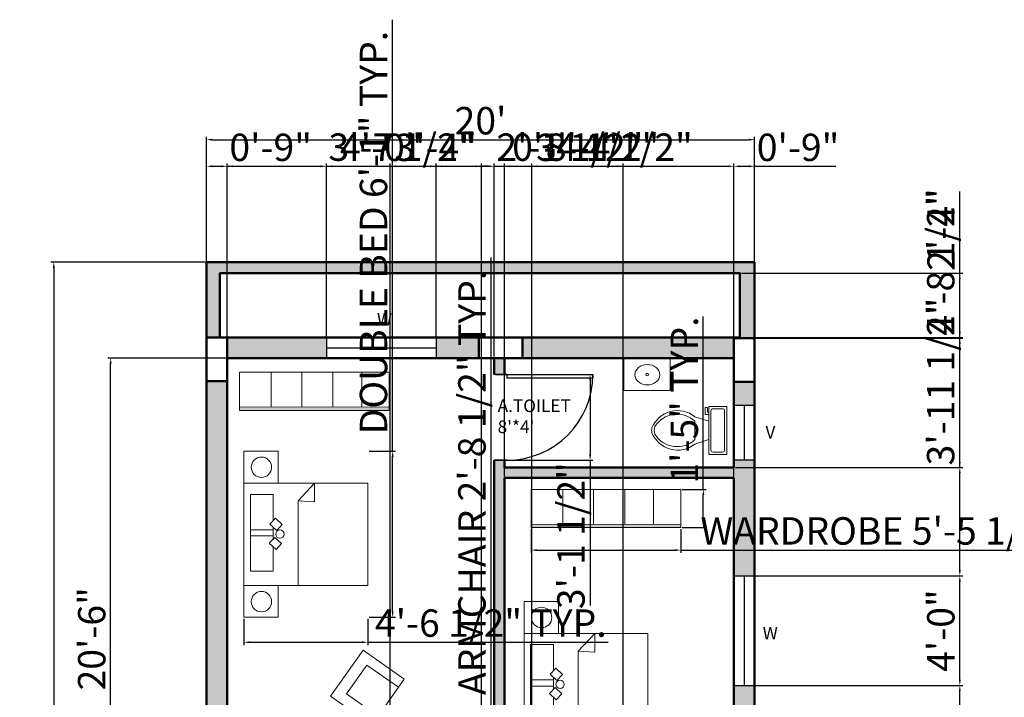
# Model space of a CAD drawing. Units: inches. Extents: x 2063 to 3370, y 2091 to 2971.
# Tile 7 of 14: x 2063 to 2494, y 2674 to 2971. Entities that reach past the tile are written whole.
import ezdxf

# ---------------------------------------------------------------- set-up
doc = ezdxf.new("R2010")
doc.units = ezdxf.units.IN
for name, color, linetype, lineweight in [('A-ANNO-DIMS', 2, 'Continuous', 18), ('A-ANNO-TEXT', 7, 'Continuous', 18), ('A-AREA-IDEN', 3, 'Continuous', 18), ('A-COLS', 7, 'Continuous', 50), ('A-DOOR', 4, 'Continuous', 25), ('A-FLOR-FIXT', 9, 'Continuous', 18), ('A-FURN', 8, 'Continuous', 18), ('A-GLAZ', 131, 'Continuous', 25), ('A-WALL', 7, 'Continuous', 50), ('A-WALL-PATT', 8, 'Continuous', 13)]:
    doc.layers.add(name, color=color, linetype=linetype, lineweight=lineweight)
doc.styles.get("Standard").update_dxf_attribs({"font": 'arial.ttf'})
doc.dimstyles.new('ISO-25', dxfattribs={"dimtxt": 12, "dimasz": 2.5, "dimexe": 1.25, "dimexo": 0.625, "dimtad": 1, "dimdec": 0, "dimlunit": 4, "dimtxsty": 'Standard', "dimcen": 2.5, "dimadec": 0, "dimazin": 0, "dimtfac": 1, "dimtdec": 0, "dimtmove": 0, "dimatfit": 3, "dimfxl": 1, "dimarcsym": 0})

# ---------------------------------------------------------------- blocks, each defined once
blk = doc.blocks.new('*U2')
for p, q in [((0, 0), (0, -6)), ((40, 0), (40, -6))]:
    blk.add_line(p, q)
blk.add_lwpolyline([(0, 0), (0, 40), (1.75, 40), (1.75, 0)], close=True)
blk.add_arc((0, 0), 40, 0, 90)
blk = doc.blocks.new('*U4')
for p, q in [((9.5, -6), (9.5, -2)), ((-10, -8.5), (-8, -8.5)), ((-10, -9.5), (-10, -8.5)), ((-8, -8.5), (-8, -8)), ((-7, -8), (-7, -9.5)), ((-4, -8), (-6, -14)), ((4, -8), (6, -14)), ((-7, -9.5), (-10, -9.5)), ((4, -14), (-4, -14))]:
    blk.add_line(p, q)
blk.add_lwpolyline([(10.5, -8), (10.5, 0), (-10.5, 0), (-10.5, -8)], close=True)
for points in [[(-9.5, -2), (-9.5, -6)], [(8.5, -1), (-8.5, -1)], [(-8.5, -7), (8.5, -7)]]:
    blk.add_lwpolyline(points)
for centre, radius, start, end in [((-8.62, -1.88), 0.884, 81.8699, 188.1301), ((8.62, -1.88), 0.884, 351.8699, 98.1301), ((-8.62, -6.12), 0.884, 171.8699, 278.1301), ((8.62, -6.12), 0.884, 261.8699, 8.1301), ((3.52, -21.58), 12.17, 141.4691, 247.9714), ((4.2, -21.82), 11.33, 136.3677, 238.9468), ((-3.52, -21.58), 12.17, 292.0284, 38.5307), ((-4.2, -21.82), 11.33, 301.053, 43.6321), ((0, -27.88), 4, 245.7318, 294.2682), ((0, -29), 4, 254.8605, 285.1395)]:
    blk.add_arc(centre, radius, start, end)
blk = doc.blocks.new('*D5')
at = {"layer": 'A-ANNO-DIMS', "color": 0, "lineweight": -2, "transparency": 16777216}
for p, q in [((2144.72, 2865.05), (2144.72, 2919.33)), ((2147.22, 2918.08), (2382.22, 2918.08)), ((2384.72, 2865.05), (2384.72, 2919.33))]:
    blk.add_line(p, q, dxfattribs=at)
at = {"layer": 'A-ANNO-DIMS', "color": 0, "transparency": 16777216}
for points in [[(2147.22, 2918.5), (2147.22, 2917.67), (2144.72, 2918.08)], [(2382.22, 2918.5), (2382.22, 2917.67), (2384.72, 2918.08)]]:
    blk.add_solid(points, dxfattribs=at)
at = {"layer": 'Defpoints', "color": 0, "transparency": 16777216}
for p in [(2384.72, 2918.08), (2144.72, 2864.43), (2384.72, 2864.43)]:
    blk.add_point(p, dxfattribs=at)
at = {"layer": 'A-ANNO-DIMS', "color": 0, "transparency": 16777216, "insert": (2264.72, 2924.84), "char_height": 12, "attachment_point": 5}
blk.add_mtext("20'", dxfattribs=at)
blk = doc.blocks.new('*D6')
at = {"layer": 'A-ANNO-DIMS', "color": 0, "lineweight": -2, "transparency": 16777216}
for p, q in [((2144.1, 2864.43), (2076.56, 2864.43)), ((2077.81, 2861.93), (2077.81, 2146.93)), ((2144.1, 2144.43), (2076.56, 2144.43))]:
    blk.add_line(p, q, dxfattribs=at)
at = {"layer": 'A-ANNO-DIMS', "color": 0, "transparency": 16777216}
for points in [[(2077.39, 2861.93), (2078.23, 2861.93), (2077.81, 2864.43)], [(2077.39, 2146.93), (2078.23, 2146.93), (2077.81, 2144.43)]]:
    blk.add_solid(points, dxfattribs=at)
at = {"layer": 'Defpoints', "color": 0, "transparency": 16777216}
for p in [(2144.72, 2864.43), (2077.81, 2144.43), (2144.72, 2144.43)]:
    blk.add_point(p, dxfattribs=at)
at = {"layer": 'A-ANNO-DIMS', "color": 0, "transparency": 16777216, "insert": (2071.06, 2504.43), "char_height": 12, "attachment_point": 5, "rotation": 90}
blk.add_mtext("60'", dxfattribs=at)
blk = doc.blocks.new('BED-DOUBLE')
for p, q in [((23.79, 50.98), (30.96, 58.78)), ((30.96, 58.78), (30.96, 50.54)), ((23.79, 14), (23.79, 50.98)), ((30.96, 50.54), (23.79, 50.98))]:
    blk.add_line(p, q)
for points in [[(0, 58.78), (15.11, 58.78), (15.11, 72.78), (0, 72.78)], [(0, 58.78), (54.26, 58.78), (54.26, 14), (0, 14)], [(11.45, 40.86), (13.89, 43.46), (16.84, 40.71), (14.4, 38.1)], [(11.16, 32.43), (13.59, 35.03), (16.54, 32.28), (14.11, 29.67)], [(0, 0), (15.11, 0), (15.11, 14), (0, 14)]]:
    blk.add_lwpolyline(points, close=True)
for points in [[(12.88, 42.39), (12.88, 53.87), (2.9, 53.87), (2.9, 35.71), (12.88, 35.71), (12.88, 39.52)], [(12.88, 34.27), (12.88, 38.39), (2.9, 38.39), (2.9, 20.23), (12.88, 20.23), (12.88, 30.81)]]:
    blk.add_lwpolyline(points)
for centre, radius in [((7.71, 65.74), 4.47), ((15.81, 36.46), 1.81), ((7.71, 6.86), 4.47)]:
    blk.add_circle(centre, radius)
blk = doc.blocks.new('WARDROBE')
for p, q in [((13.88, 1.44), (13.88, 16.75)), ((27.33, 1.44), (27.33, 16.75)), ((40.97, 1.44), (40.97, 16.75)), ((53.56, 1.44), (53.56, 16.75)), ((0, 1.42), (65.55, 1.52))]:
    blk.add_line(p, q)
blk.add_lwpolyline([(0, 16.75), (65.55, 16.75), (65.55, 0), (0, 0)], close=True)
blk = doc.blocks.new('ARMCHAIR')
for p, q in [((10.7, 28.87), (13.03, 32.61)), ((13.03, 32.61), (31.78, 20.96)), ((0, 11.65), (3.54, 17.35)), ((31.78, 20.96), (18.75, 0)), ((18.75, 0), (0, 11.65))]:
    blk.add_line(p, q)
blk.add_lwpolyline([(2.55, 15.75), (16.92, 6.82), (25.07, 19.93), (10.7, 28.87)], close=True)
blk = doc.blocks.new('*D20')
at = {"layer": 'A-ANNO-DIMS', "color": 0, "lineweight": -2, "transparency": 16777216}
for p, q in [((2226.23, 2781.63), (2226.23, 2970.65)), ((2215.94, 2781.63), (2227.48, 2781.63)), ((2226.23, 2711.35), (2226.23, 2779.13)), ((2215.94, 2708.85), (2227.48, 2708.85))]:
    blk.add_line(p, q, dxfattribs=at)
at = {"layer": 'A-ANNO-DIMS', "color": 0, "transparency": 16777216}
for points in [[(2225.81, 2779.13), (2226.65, 2779.13), (2226.23, 2781.63)], [(2225.81, 2711.35), (2226.65, 2711.35), (2226.23, 2708.85)]]:
    blk.add_solid(points, dxfattribs=at)
at = {"layer": 'Defpoints', "color": 0, "transparency": 16777216}
for p in [(2215.31, 2781.63), (2226.23, 2781.63), (2215.31, 2708.85)]:
    blk.add_point(p, dxfattribs=at)
at = {"layer": 'A-ANNO-DIMS', "color": 0, "transparency": 16777216, "insert": (2219.4, 2877.39), "char_height": 12, "attachment_point": 5, "rotation": 90}
blk.add_mtext('DOUBLE BED 6\'-1" TYP.', dxfattribs=at)
blk = doc.blocks.new('*D21')
at = {"layer": 'A-ANNO-DIMS', "color": 0, "lineweight": -2, "transparency": 16777216}
for p, q in [((2161.05, 2708.22), (2161.05, 2696.68)), ((2215.31, 2708.22), (2215.31, 2696.68)), ((2163.55, 2697.93), (2212.81, 2697.93)), ((2215.31, 2697.93), (2320.65, 2697.93))]:
    blk.add_line(p, q, dxfattribs=at)
at = {"layer": 'A-ANNO-DIMS', "color": 0, "transparency": 16777216}
for points in [[(2163.55, 2698.35), (2163.55, 2697.51), (2161.05, 2697.93)], [(2212.81, 2698.35), (2212.81, 2697.51), (2215.31, 2697.93)]]:
    blk.add_solid(points, dxfattribs=at)
at = {"layer": 'Defpoints', "color": 0, "transparency": 16777216}
for p in [(2161.05, 2708.85), (2215.31, 2708.85), (2215.31, 2697.93)]:
    blk.add_point(p, dxfattribs=at)
at = {"layer": 'A-ANNO-DIMS', "color": 0, "transparency": 16777216, "insert": (2269.23, 2704.76), "char_height": 12, "attachment_point": 5}
blk.add_mtext('4\'-6 1/2" TYP.', dxfattribs=at)
blk = doc.blocks.new('*D22')
at = {"layer": 'A-ANNO-DIMS', "color": 0, "lineweight": -2, "transparency": 16777216}
for p, q in [((2286.92, 2747.51), (2286.92, 2737.05)), ((2352.47, 2747.51), (2352.47, 2737.05)), ((2289.42, 2738.3), (2349.97, 2738.3)), ((2352.47, 2738.3), (2561.2, 2738.3))]:
    blk.add_line(p, q, dxfattribs=at)
at = {"layer": 'A-ANNO-DIMS', "color": 0, "transparency": 16777216}
for points in [[(2289.42, 2738.72), (2289.42, 2737.89), (2286.92, 2738.3)], [(2349.97, 2738.72), (2349.97, 2737.89), (2352.47, 2738.3)]]:
    blk.add_solid(points, dxfattribs=at)
at = {"layer": 'Defpoints', "color": 0, "transparency": 16777216}
for p in [(2286.92, 2748.13), (2352.47, 2748.13), (2352.47, 2738.3)]:
    blk.add_point(p, dxfattribs=at)
at = {"layer": 'A-ANNO-DIMS', "color": 0, "transparency": 16777216, "insert": (2458.09, 2745.14), "char_height": 12, "attachment_point": 5}
blk.add_mtext('WARDROBE 5\'-5 1/2" TYP.', dxfattribs=at)
blk = doc.blocks.new('*D23')
at = {"layer": 'A-ANNO-DIMS', "color": 0, "lineweight": -2, "transparency": 16777216}
for p, q in [((2362.3, 2764.89), (2362.3, 2840.66)), ((2353.09, 2764.89), (2363.55, 2764.89)), ((2362.3, 2750.63), (2362.3, 2762.39)), ((2353.09, 2748.13), (2363.55, 2748.13))]:
    blk.add_line(p, q, dxfattribs=at)
at = {"layer": 'A-ANNO-DIMS', "color": 0, "transparency": 16777216}
for points in [[(2361.88, 2762.39), (2362.72, 2762.39), (2362.3, 2764.89)], [(2361.88, 2750.63), (2362.72, 2750.63), (2362.3, 2748.13)]]:
    blk.add_solid(points, dxfattribs=at)
at = {"layer": 'Defpoints', "color": 0, "transparency": 16777216}
for p in [(2352.47, 2764.89), (2362.3, 2764.89), (2352.47, 2748.13)]:
    blk.add_point(p, dxfattribs=at)
at = {"layer": 'A-ANNO-DIMS', "color": 0, "transparency": 16777216, "insert": (2355.55, 2804.02), "char_height": 12, "attachment_point": 5, "rotation": 90}
blk.add_mtext('1\'-5" TYP.', dxfattribs=at)
blk = doc.blocks.new('*D24')
at = {"layer": 'A-ANNO-DIMS', "color": 0, "lineweight": -2, "transparency": 16777216}
for p, q in [((2269.34, 2666.87), (2269.34, 2866.5)), ((2265.08, 2666.87), (2270.59, 2666.87)), ((2269.34, 2636.76), (2269.34, 2664.37)), ((2265.08, 2634.26), (2270.59, 2634.26))]:
    blk.add_line(p, q, dxfattribs=at)
at = {"layer": 'A-ANNO-DIMS', "color": 0, "transparency": 16777216}
for points in [[(2268.93, 2664.37), (2269.76, 2664.37), (2269.34, 2666.87)], [(2268.93, 2636.76), (2269.76, 2636.76), (2269.34, 2634.26)]]:
    blk.add_solid(points, dxfattribs=at)
at = {"layer": 'Defpoints', "color": 0, "transparency": 16777216}
for p in [(2264.45, 2666.87), (2269.34, 2666.87), (2264.45, 2634.26)]:
    blk.add_point(p, dxfattribs=at)
at = {"layer": 'A-ANNO-DIMS', "color": 0, "transparency": 16777216, "insert": (2262.51, 2767.94), "char_height": 12, "attachment_point": 5, "rotation": 90}
blk.add_mtext('ARMCHAIR 2\'-8 1/2" TYP.', dxfattribs=at)
blk = doc.blocks.new('*D32')
at = {"layer": 'A-ANNO-DIMS', "color": 0, "lineweight": -2, "transparency": 16777216}
for p, q in [((2144.72, 2832.05), (2144.72, 2907.68)), ((2153.72, 2823.05), (2153.72, 2907.68)), ((2147.22, 2906.43), (2151.22, 2906.43)), ((2153.72, 2906.43), (2189.37, 2906.43))]:
    blk.add_line(p, q, dxfattribs=at)
at = {"layer": 'A-ANNO-DIMS', "color": 0, "transparency": 16777216}
for points in [[(2147.22, 2906.84), (2147.22, 2906.01), (2144.72, 2906.43)], [(2151.22, 2906.84), (2151.22, 2906.01), (2153.72, 2906.43)]]:
    blk.add_solid(points, dxfattribs=at)
at = {"layer": 'Defpoints', "color": 0, "transparency": 16777216}
for p in [(2153.72, 2906.43), (2144.72, 2831.43), (2153.72, 2822.43)]:
    blk.add_point(p, dxfattribs=at)
at = {"layer": 'A-ANNO-DIMS', "color": 0, "transparency": 16777216, "insert": (2172.8, 2913.18), "char_height": 12, "attachment_point": 5}
blk.add_mtext('0\'-9"', dxfattribs=at)
blk = doc.blocks.new('*D33')
at = {"layer": 'A-ANNO-DIMS', "color": 0, "lineweight": -2, "transparency": 16777216}
for p, q in [((2153.72, 2823.05), (2153.72, 2907.68)), ((2197.25, 2832.05), (2197.25, 2907.68)), ((2156.22, 2906.43), (2194.75, 2906.43)), ((2197.25, 2906.43), (2260.85, 2906.43))]:
    blk.add_line(p, q, dxfattribs=at)
at = {"layer": 'A-ANNO-DIMS', "color": 0, "transparency": 16777216}
for points in [[(2156.22, 2906.84), (2156.22, 2906.01), (2153.72, 2906.43)], [(2194.75, 2906.84), (2194.75, 2906.01), (2197.25, 2906.43)]]:
    blk.add_solid(points, dxfattribs=at)
at = {"layer": 'Defpoints', "color": 0, "transparency": 16777216}
for p in [(2197.25, 2906.43), (2197.25, 2831.43), (2153.72, 2822.43)]:
    blk.add_point(p, dxfattribs=at)
at = {"layer": 'A-ANNO-DIMS', "color": 0, "transparency": 16777216, "insert": (2230.3, 2913.26), "char_height": 12, "attachment_point": 5}
blk.add_mtext('3\'-7 1/2"', dxfattribs=at)
blk = doc.blocks.new('*D34')
at = {"layer": 'A-ANNO-DIMS', "color": 0, "lineweight": -2, "transparency": 16777216}
for p, q in [((2197.25, 2832.05), (2197.25, 2907.68)), ((2245.25, 2832.05), (2245.25, 2907.68)), ((2199.75, 2906.43), (2242.75, 2906.43))]:
    blk.add_line(p, q, dxfattribs=at)
at = {"layer": 'A-ANNO-DIMS', "color": 0, "transparency": 16777216}
for points in [[(2199.75, 2906.84), (2199.75, 2906.01), (2197.25, 2906.43)], [(2242.75, 2906.84), (2242.75, 2906.01), (2245.25, 2906.43)]]:
    blk.add_solid(points, dxfattribs=at)
at = {"layer": 'Defpoints', "color": 0, "transparency": 16777216}
for p in [(2245.25, 2906.43), (2197.25, 2831.43), (2245.25, 2831.43)]:
    blk.add_point(p, dxfattribs=at)
at = {"layer": 'A-ANNO-DIMS', "color": 0, "transparency": 16777216, "insert": (2221.25, 2913.18), "char_height": 12, "attachment_point": 5}
blk.add_mtext('4\'-0"', dxfattribs=at)
blk = doc.blocks.new('*D35')
at = {"layer": 'A-ANNO-DIMS', "color": 0, "lineweight": -2, "transparency": 16777216}
for p, q in [((2245.25, 2832.05), (2245.25, 2907.68)), ((2270.72, 2823.05), (2270.72, 2907.68)), ((2247.75, 2906.43), (2268.22, 2906.43)), ((2270.72, 2906.43), (2334.54, 2906.43))]:
    blk.add_line(p, q, dxfattribs=at)
at = {"layer": 'A-ANNO-DIMS', "color": 0, "transparency": 16777216}
for points in [[(2247.75, 2906.84), (2247.75, 2906.01), (2245.25, 2906.43)], [(2268.22, 2906.84), (2268.22, 2906.01), (2270.72, 2906.43)]]:
    blk.add_solid(points, dxfattribs=at)
at = {"layer": 'Defpoints', "color": 0, "transparency": 16777216}
for p in [(2270.72, 2906.43), (2245.25, 2831.43), (2270.72, 2822.43)]:
    blk.add_point(p, dxfattribs=at)
at = {"layer": 'A-ANNO-DIMS', "color": 0, "transparency": 16777216, "insert": (2303.88, 2913.26), "char_height": 12, "attachment_point": 5}
blk.add_mtext('2\'-1 1/2"', dxfattribs=at)
blk = doc.blocks.new('*D36')
at = {"layer": 'A-ANNO-DIMS', "color": 0, "lineweight": -2, "transparency": 16777216}
for p, q in [((2270.72, 2823.05), (2270.72, 2907.68)), ((2275.22, 2823.05), (2275.22, 2907.68)), ((2268.22, 2906.43), (2265.72, 2906.43)), ((2270.72, 2906.43), (2275.22, 2906.43)), ((2277.72, 2906.43), (2341.33, 2906.43))]:
    blk.add_line(p, q, dxfattribs=at)
at = {"layer": 'A-ANNO-DIMS', "color": 0, "transparency": 16777216}
for points in [[(2268.22, 2906.84), (2268.22, 2906.01), (2270.72, 2906.43)], [(2277.72, 2906.84), (2277.72, 2906.01), (2275.22, 2906.43)]]:
    blk.add_solid(points, dxfattribs=at)
at = {"layer": 'Defpoints', "color": 0, "transparency": 16777216}
for p in [(2275.22, 2906.43), (2270.72, 2822.43), (2275.22, 2822.43)]:
    blk.add_point(p, dxfattribs=at)
at = {"layer": 'A-ANNO-DIMS', "color": 0, "transparency": 16777216, "insert": (2310.78, 2913.26), "char_height": 12, "attachment_point": 5}
blk.add_mtext('0\'-4 1/2"', dxfattribs=at)
blk = doc.blocks.new('*D37')
at = {"layer": 'A-ANNO-DIMS', "color": 0, "lineweight": -2, "transparency": 16777216}
for p, q in [((2275.22, 2770.55), (2275.22, 2907.68)), ((2375.72, 2770.55), (2375.72, 2907.68)), ((2277.72, 2906.43), (2373.22, 2906.43))]:
    blk.add_line(p, q, dxfattribs=at)
at = {"layer": 'A-ANNO-DIMS', "color": 0, "transparency": 16777216}
for points in [[(2277.72, 2906.84), (2277.72, 2906.01), (2275.22, 2906.43)], [(2373.22, 2906.84), (2373.22, 2906.01), (2375.72, 2906.43)]]:
    blk.add_solid(points, dxfattribs=at)
at = {"layer": 'Defpoints', "color": 0, "transparency": 16777216}
for p in [(2375.72, 2906.43), (2275.22, 2769.93), (2375.72, 2769.93)]:
    blk.add_point(p, dxfattribs=at)
at = {"layer": 'A-ANNO-DIMS', "color": 0, "transparency": 16777216, "insert": (2325.47, 2913.26), "char_height": 12, "attachment_point": 5}
blk.add_mtext('8\'-4 1/2"', dxfattribs=at)
blk = doc.blocks.new('*D38')
at = {"layer": 'A-ANNO-DIMS', "color": 0, "lineweight": -2, "transparency": 16777216}
for p, q in [((2375.72, 2823.05), (2375.72, 2907.68)), ((2384.72, 2831.77), (2384.72, 2907.68)), ((2378.22, 2906.43), (2382.22, 2906.43)), ((2384.72, 2906.43), (2420.37, 2906.43))]:
    blk.add_line(p, q, dxfattribs=at)
at = {"layer": 'A-ANNO-DIMS', "color": 0, "transparency": 16777216}
for points in [[(2378.22, 2906.84), (2378.22, 2906.01), (2375.72, 2906.43)], [(2382.22, 2906.84), (2382.22, 2906.01), (2384.72, 2906.43)]]:
    blk.add_solid(points, dxfattribs=at)
at = {"layer": 'Defpoints', "color": 0, "transparency": 16777216}
for p in [(2384.72, 2906.43), (2384.72, 2831.15), (2375.72, 2822.43)]:
    blk.add_point(p, dxfattribs=at)
at = {"layer": 'A-ANNO-DIMS', "color": 0, "transparency": 16777216, "insert": (2403.8, 2913.18), "char_height": 12, "attachment_point": 5}
blk.add_mtext('0\'-9"', dxfattribs=at)
blk = doc.blocks.new('*D58')
at = {"layer": 'A-ANNO-DIMS', "color": 0, "lineweight": -2, "transparency": 16777216}
for p, q in [((2153.1, 2822.43), (2101.47, 2822.43)), ((2102.72, 2578.93), (2102.72, 2819.93)), ((2153.1, 2576.43), (2101.47, 2576.43))]:
    blk.add_line(p, q, dxfattribs=at)
at = {"layer": 'A-ANNO-DIMS', "color": 0, "transparency": 16777216}
for points in [[(2102.31, 2819.93), (2103.14, 2819.93), (2102.72, 2822.43)], [(2102.31, 2578.93), (2103.14, 2578.93), (2102.72, 2576.43)]]:
    blk.add_solid(points, dxfattribs=at)
at = {"layer": 'Defpoints', "color": 0, "transparency": 16777216}
for p in [(2102.72, 2822.43), (2153.72, 2822.43), (2153.72, 2576.43)]:
    blk.add_point(p, dxfattribs=at)
at = {"layer": 'A-ANNO-DIMS', "color": 0, "transparency": 16777216, "insert": (2095.97, 2699.43), "char_height": 12, "attachment_point": 5, "rotation": 90}
blk.add_mtext('20\'-6"', dxfattribs=at)
blk = doc.blocks.new('*D65')
at = {"layer": 'A-ANNO-DIMS', "color": 0, "lineweight": -2, "transparency": 16777216}
for p, q in [((2376.35, 2679.03), (2475.9, 2679.03)), ((2474.65, 2578.93), (2474.65, 2676.53)), ((2376.35, 2576.43), (2475.9, 2576.43))]:
    blk.add_line(p, q, dxfattribs=at)
at = {"layer": 'A-ANNO-DIMS', "color": 0, "transparency": 16777216}
for points in [[(2474.23, 2676.53), (2475.06, 2676.53), (2474.65, 2679.03)], [(2474.23, 2578.93), (2475.06, 2578.93), (2474.65, 2576.43)]]:
    blk.add_solid(points, dxfattribs=at)
at = {"layer": 'Defpoints', "color": 0, "transparency": 16777216}
for p in [(2375.72, 2679.03), (2474.65, 2679.03), (2375.72, 2576.43)]:
    blk.add_point(p, dxfattribs=at)
at = {"layer": 'A-ANNO-DIMS', "color": 0, "transparency": 16777216, "insert": (2467.82, 2627.73), "char_height": 12, "attachment_point": 5, "rotation": 90}
blk.add_mtext('8\'-6 1/2"', dxfattribs=at)
blk = doc.blocks.new('*D66')
at = {"layer": 'A-ANNO-DIMS', "color": 0, "lineweight": -2, "transparency": 16777216}
for p, q in [((2376.35, 2727.03), (2475.9, 2727.03)), ((2474.65, 2681.53), (2474.65, 2724.53)), ((2376.35, 2679.03), (2475.9, 2679.03))]:
    blk.add_line(p, q, dxfattribs=at)
at = {"layer": 'A-ANNO-DIMS', "color": 0, "transparency": 16777216}
for points in [[(2474.23, 2724.53), (2475.06, 2724.53), (2474.65, 2727.03)], [(2474.23, 2681.53), (2475.06, 2681.53), (2474.65, 2679.03)]]:
    blk.add_solid(points, dxfattribs=at)
at = {"layer": 'Defpoints', "color": 0, "transparency": 16777216}
for p in [(2375.72, 2727.03), (2474.65, 2727.03), (2375.72, 2679.03)]:
    blk.add_point(p, dxfattribs=at)
at = {"layer": 'A-ANNO-DIMS', "color": 0, "transparency": 16777216, "insert": (2467.89, 2703.03), "char_height": 12, "attachment_point": 5, "rotation": 90}
blk.add_mtext('4\'-0"', dxfattribs=at)
blk = doc.blocks.new('*D67')
at = {"layer": 'A-ANNO-DIMS', "color": 0, "lineweight": -2, "transparency": 16777216}
for p, q in [((2474.65, 2774.43), (2474.65, 2847.35)), ((2376.35, 2774.43), (2475.9, 2774.43)), ((2474.65, 2729.53), (2474.65, 2771.93)), ((2376.35, 2727.03), (2475.9, 2727.03))]:
    blk.add_line(p, q, dxfattribs=at)
at = {"layer": 'A-ANNO-DIMS', "color": 0, "transparency": 16777216}
for points in [[(2474.23, 2771.93), (2475.06, 2771.93), (2474.65, 2774.43)], [(2474.23, 2729.53), (2475.06, 2729.53), (2474.65, 2727.03)]]:
    blk.add_solid(points, dxfattribs=at)
at = {"layer": 'Defpoints', "color": 0, "transparency": 16777216}
for p in [(2375.72, 2774.43), (2474.65, 2774.43), (2375.72, 2727.03)]:
    blk.add_point(p, dxfattribs=at)
at = {"layer": 'A-ANNO-DIMS', "color": 0, "transparency": 16777216, "insert": (2467.81, 2812.14), "char_height": 12, "attachment_point": 5, "rotation": 90}
blk.add_mtext('3\'-11 1/2"', dxfattribs=at)
blk = doc.blocks.new('*D68')
at = {"layer": 'A-ANNO-DIMS', "color": 0, "lineweight": -2, "transparency": 16777216}
for p, q in [((2474.65, 2831.15), (2474.65, 2895.24)), ((2376.35, 2831.15), (2475.9, 2831.15)), ((2474.65, 2776.93), (2474.65, 2828.65)), ((2376.35, 2774.43), (2475.9, 2774.43))]:
    blk.add_line(p, q, dxfattribs=at)
at = {"layer": 'A-ANNO-DIMS', "color": 0, "transparency": 16777216}
for points in [[(2474.23, 2828.65), (2475.06, 2828.65), (2474.65, 2831.15)], [(2474.23, 2776.93), (2475.06, 2776.93), (2474.65, 2774.43)]]:
    blk.add_solid(points, dxfattribs=at)
at = {"layer": 'Defpoints', "color": 0, "transparency": 16777216}
for p in [(2375.72, 2831.15), (2474.65, 2831.15), (2375.72, 2774.43)]:
    blk.add_point(p, dxfattribs=at)
at = {"layer": 'A-ANNO-DIMS', "color": 0, "transparency": 16777216, "insert": (2467.82, 2864.44), "char_height": 12, "attachment_point": 5, "rotation": 90}
blk.add_mtext('4\'-8 1/2"', dxfattribs=at)
blk = doc.blocks.new('*D69')
at = {"layer": 'A-ANNO-DIMS', "color": 0, "lineweight": -2, "transparency": 16777216}
for p, q in [((2474.65, 2859.54), (2474.65, 2895.4)), ((2378.96, 2859.54), (2475.9, 2859.54)), ((2474.65, 2833.93), (2474.65, 2857.04)), ((2378.96, 2831.43), (2475.9, 2831.43))]:
    blk.add_line(p, q, dxfattribs=at)
at = {"layer": 'A-ANNO-DIMS', "color": 0, "transparency": 16777216}
for points in [[(2474.23, 2857.04), (2475.06, 2857.04), (2474.65, 2859.54)], [(2474.23, 2833.93), (2475.06, 2833.93), (2474.65, 2831.43)]]:
    blk.add_solid(points, dxfattribs=at)
at = {"layer": 'Defpoints', "color": 0, "transparency": 16777216}
for p in [(2378.34, 2859.54), (2474.65, 2859.54), (2378.34, 2831.43)]:
    blk.add_point(p, dxfattribs=at)
at = {"layer": 'A-ANNO-DIMS', "color": 0, "transparency": 16777216, "insert": (2468, 2878.72), "char_height": 12, "attachment_point": 5, "rotation": 90}
blk.add_mtext('2\'-4"', dxfattribs=at)
blk = doc.blocks.new('*D72')
at = {"layer": 'A-ANNO-DIMS', "color": 0, "lineweight": -2, "transparency": 16777216}
for p, q in [((2225.08, 2577.05), (2225.08, 2907.68)), ((2265.08, 2572.55), (2265.08, 2907.68)), ((2227.58, 2906.43), (2262.58, 2906.43))]:
    blk.add_line(p, q, dxfattribs=at)
at = {"layer": 'A-ANNO-DIMS', "color": 0, "transparency": 16777216}
for points in [[(2227.58, 2906.84), (2227.58, 2906.01), (2225.08, 2906.43)], [(2262.58, 2906.84), (2262.58, 2906.01), (2265.08, 2906.43)]]:
    blk.add_solid(points, dxfattribs=at)
at = {"layer": 'Defpoints', "color": 0, "transparency": 16777216}
for p in [(2265.08, 2906.43), (2225.08, 2576.43), (2265.08, 2571.93)]:
    blk.add_point(p, dxfattribs=at)
at = {"layer": 'A-ANNO-DIMS', "color": 0, "transparency": 16777216, "insert": (2245.08, 2913.18), "char_height": 12, "attachment_point": 5}
blk.add_mtext('3\'-4"', dxfattribs=at)
blk = doc.blocks.new('*D73')
at = {"layer": 'A-ANNO-DIMS', "color": 0, "lineweight": -2, "transparency": 16777216}
for p, q in [((2287.14, 2572.55), (2287.14, 2907.68)), ((2327.14, 2577.05), (2327.14, 2907.68)), ((2289.64, 2906.43), (2324.64, 2906.43))]:
    blk.add_line(p, q, dxfattribs=at)
at = {"layer": 'A-ANNO-DIMS', "color": 0, "transparency": 16777216}
for points in [[(2289.64, 2906.84), (2289.64, 2906.01), (2287.14, 2906.43)], [(2324.64, 2906.84), (2324.64, 2906.01), (2327.14, 2906.43)]]:
    blk.add_solid(points, dxfattribs=at)
at = {"layer": 'Defpoints', "color": 0, "transparency": 16777216}
for p in [(2327.14, 2906.43), (2327.14, 2576.43), (2287.14, 2571.93)]:
    blk.add_point(p, dxfattribs=at)
at = {"layer": 'A-ANNO-DIMS', "color": 0, "transparency": 16777216, "insert": (2307.14, 2913.18), "char_height": 12, "attachment_point": 5}
blk.add_mtext('3\'-4"', dxfattribs=at)
blk = doc.blocks.new('*D74')
at = {"layer": 'A-ANNO-DIMS', "color": 0, "lineweight": -2, "transparency": 16777216}
for p, q in [((2271.35, 2815.29), (2313.97, 2815.29)), ((2312.72, 2812.79), (2312.72, 2780.18)), ((2271.35, 2777.68), (2313.97, 2777.68)), ((2312.72, 2777.68), (2312.72, 2714.08))]:
    blk.add_line(p, q, dxfattribs=at)
at = {"layer": 'A-ANNO-DIMS', "color": 0, "transparency": 16777216}
for points in [[(2312.31, 2812.79), (2313.14, 2812.79), (2312.72, 2815.29)], [(2312.31, 2780.18), (2313.14, 2780.18), (2312.72, 2777.68)]]:
    blk.add_solid(points, dxfattribs=at)
at = {"layer": 'Defpoints', "color": 0, "transparency": 16777216}
for p in [(2270.72, 2815.29), (2270.72, 2777.68), (2312.72, 2777.68)]:
    blk.add_point(p, dxfattribs=at)
at = {"layer": 'A-ANNO-DIMS', "color": 0, "transparency": 16777216, "insert": (2305.89, 2744.63), "char_height": 12, "attachment_point": 5, "rotation": 90}
blk.add_mtext('3\'-1 1/2"', dxfattribs=at)

msp = doc.modelspace()

# ---------------------------------------------------------------- hatches: boundary and pattern name
at = {"layer": 'A-FURN'}
h = msp.add_hatch(color=256, dxfattribs=at)
h.dxf.hatch_style = 1
h.paths.add_polyline_path([(2224.68, 2800.98), (2159.13, 2800.89), (2159.13, 2799.47), (2224.68, 2799.47)])
h = msp.add_hatch(color=256, dxfattribs=at)
h.dxf.hatch_style = 1
h.paths.add_polyline_path([(2352.47, 2749.65), (2286.92, 2749.56), (2286.92, 2748.13), (2352.47, 2748.13)])
at = {"layer": 'A-WALL-PATT'}
h = msp.add_hatch(color=256, dxfattribs=at)
h.dxf.hatch_style = 1
h.paths.add_polyline_path([(2197.25, 2831.43), (2153.72, 2831.43), (2153.72, 2822.43), (2197.25, 2822.43)], flags=17)
h.paths.add_polyline_path([(2264.04, 2831.43), (2245.25, 2831.43), (2245.25, 2822.43), (2264.04, 2822.43)], flags=17)
h.paths.add_polyline_path([(2375.72, 2831.15), (2384.72, 2831.15), (2384.72, 2864.43), (2144.72, 2864.43), (2144.72, 2831.43), (2150.59, 2831.43), (2150.59, 2859.54), (2378.34, 2859.54), (2378.34, 2831.43), (2283.15, 2831.43), (2283.15, 2822.43), (2375.72, 2822.43)])
h = msp.add_hatch(color=256, dxfattribs=at)
h.dxf.hatch_style = 1
h.paths.add_polyline_path([(2275.22, 2822.43), (2270.72, 2822.43), (2270.72, 2815.29), (2275.22, 2815.29)])
h.paths.add_polyline_path([(2384.72, 2777.84), (2375.72, 2777.84), (2375.72, 2774.43), (2371.22, 2774.43), (2275.22, 2774.43), (2275.22, 2777.68), (2270.72, 2777.68), (2270.72, 2644.58), (2275.22, 2644.58), (2275.22, 2769.93), (2375.72, 2769.93), (2375.72, 2727.03), (2384.72, 2727.03)])
h.paths.add_polyline_path([(2384.72, 2812.03), (2375.72, 2812.03), (2375.72, 2801.84), (2384.72, 2801.84)])
h.paths.add_polyline_path([(2275.22, 2625.46), (2270.72, 2625.46), (2270.72, 2576.43), (2265.08, 2576.43), (2265.08, 2571.93), (2287.14, 2571.93), (2287.14, 2576.43), (2275.22, 2576.43)])
h = msp.add_hatch(color=256, dxfattribs=at)
h.dxf.hatch_style = 1
h.paths.add_polyline_path([(2384.72, 2679.03), (2375.72, 2679.03), (2375.72, 2645.28), (2384.72, 2645.28)])
h.paths.add_polyline_path([(2384.72, 2626.16), (2375.72, 2626.16), (2375.72, 2576.43), (2327.14, 2576.43), (2327.14, 2571.93), (2375.72, 2571.93), (2375.72, 2523.93), (2384.72, 2523.93)])
h.paths.add_polyline_path([(2384.72, 2463.93), (2375.72, 2463.93), (2375.72, 2383.04), (2384.72, 2383.04)])
h.paths.add_polyline_path([(2153.72, 2812.31), (2144.72, 2812.31), (2144.72, 2638.63), (2153.72, 2638.63)])
h.paths.add_polyline_path([(2225.08, 2576.43), (2153.72, 2576.43), (2153.72, 2619.52), (2144.72, 2619.52), (2144.72, 2420.38), (2153.72, 2420.38), (2153.72, 2466.93), (2175.31, 2466.93), (2175.31, 2471.43), (2153.72, 2471.43), (2153.72, 2519.43), (2213.72, 2519.43), (2213.72, 2507.47), (2214.09, 2507.47), (2218.22, 2507.47), (2218.22, 2519.43), (2218.22, 2523.93), (2218.22, 2529.53), (2213.72, 2529.53), (2213.72, 2523.93), (2153.72, 2523.93), (2153.72, 2571.93), (2213.72, 2571.93), (2213.72, 2563.16), (2218.22, 2563.16), (2218.22, 2571.93), (2225.08, 2571.93)])

# ---------------------------------------------------------------- linework, layer by layer
at = {"layer": 'A-COLS'}
for points in [[(2144.72, 2831.43), (2153.72, 2831.43), (2153.72, 2812.31), (2144.72, 2812.31)], [(2264.04, 2822.43), (2264.04, 2831.43), (2283.15, 2831.43), (2283.15, 2822.43)], [(2375.72, 2831.15), (2384.72, 2831.15), (2384.72, 2812.03), (2375.72, 2812.03)]]:
    msp.add_lwpolyline(points, close=True, dxfattribs=at)
at = {"layer": 'A-FLOR-FIXT'}
msp.add_lwpolyline([(2327.54, 2808.22), (2347.83, 2808.22), (2347.83, 2822.43), (2327.54, 2822.43)], close=True, dxfattribs=at)
msp.add_circle((2337.67, 2815.16), 0.596, dxfattribs=at)
msp.add_ellipse((2337.79, 2815.13), major_axis=(5.46, 0), ratio=0.818182, dxfattribs=at)
at = {"layer": 'A-GLAZ'}
for p, q in [((2197.25, 2831.43), (2197.25, 2822.43)), ((2245.25, 2831.43), (2245.25, 2822.43)), ((2197.25, 2826.93), (2245.25, 2826.93)), ((2375.72, 2801.84), (2384.72, 2801.84)), ((2380.22, 2801.84), (2380.22, 2777.84)), ((2375.72, 2777.84), (2384.72, 2777.84)), ((2375.72, 2727.03), (2384.72, 2727.03)), ((2380.22, 2727.03), (2380.22, 2679.03)), ((2375.72, 2679.03), (2384.72, 2679.03))]:
    msp.add_line(p, q, dxfattribs=at)
at = {"layer": 'A-WALL'}
for p, q in [((2153.72, 2822.43), (2270.72, 2822.43)), ((2153.72, 2822.43), (2270.72, 2822.43)), ((2270.72, 2822.43), (2270.72, 2815.29)), ((2275.22, 2822.43), (2275.22, 2815.29)), ((2275.22, 2822.43), (2275.22, 2815.29)), ((2275.22, 2822.43), (2375.72, 2822.43)), ((2270.72, 2777.68), (2270.72, 2576.43)), ((2275.22, 2777.68), (2275.22, 2774.43)), ((2275.22, 2777.68), (2275.22, 2774.43)), ((2275.22, 2774.43), (2375.72, 2774.43)), ((2371.22, 2774.43), (2375.72, 2774.43)), ((2275.22, 2769.93), (2375.72, 2769.93)), ((2275.22, 2769.93), (2275.22, 2576.43))]:
    msp.add_line(p, q, dxfattribs=at)
for points in [[(2144.72, 2144.43), (2384.72, 2144.43), (2384.72, 2864.43), (2144.72, 2864.43)], [(2378.34, 2831.43), (2378.34, 2859.54), (2150.59, 2859.54), (2150.59, 2831.43)]]:
    msp.add_lwpolyline(points, close=True, dxfattribs=at)
for points in [[(2153.72, 2822.43), (2153.72, 2576.43)], [(2375.72, 2774.43), (2375.72, 2822.43)], [(2375.72, 2576.43), (2375.72, 2769.93)]]:
    msp.add_lwpolyline(points, dxfattribs=at)

# ---------------------------------------------------------------- block references
at = {"layer": 'A-DOOR', "xscale": 0.9400530028669262, "yscale": 0.9400530028669262, "zscale": 0.9400530028669262, "rotation": 270}
msp.add_blockref('*U2', (2276.36, 2815.29), dxfattribs=at)
at = {"layer": 'A-FLOR-FIXT', "rotation": 270}
msp.add_blockref('*U4', (2372.65, 2790.74), dxfattribs=at)
at = {"layer": 'A-FURN'}
for name, p in [('WARDROBE', (2159.13, 2799.47)), ('BED-DOUBLE', (2161.05, 2708.85)), ('WARDROBE', (2286.92, 2748.13)), ('BED-DOUBLE', (2283.77, 2643.05))]:
    msp.add_blockref(name, p, dxfattribs=at)
at = {"layer": 'A-FURN', "extrusion": (0, 0, -1), "zscale": -1, "rotation": 66.95512356980241}
msp.add_blockref('ARMCHAIR', (-2206.41, 2657.05), dxfattribs=at)

# ---------------------------------------------------------------- texts
at = {"layer": 'A-ANNO-TEXT', "char_height": 5.52, "attachment_point": 1}
for s, insert in [('W', (2219.34, 2842.22)), ('V', (2389.52, 2792.69)), ('W', (2388.32, 2704.68))]:
    msp.add_mtext_dynamic_manual_height_columns(s, width=106.0361, gutter_width=27.61, heights=[0], dxfattribs=dict(at, insert=insert))
at = {"layer": 'A-AREA-IDEN', "insert": (2272.23, 2804.28), "char_height": 5.523, "attachment_point": 1}
msp.add_mtext_dynamic_manual_height_columns("A.TOILET\\P8'*4'", width=106.0361, gutter_width=27.61, heights=[0], dxfattribs=at)

# ---------------------------------------------------------------- dimensions: what is measured, and where the dimension line sits
at = {"layer": 'A-ANNO-DIMS'}
for base, p1, p2, text, picture, middle in [((2226.23, 2781.63), (2215.31, 2708.85), (2215.31, 2781.63), 'DOUBLE BED <> TYP.', '*D20', (2219.4, 2877.39)), ((2269.34, 2666.87), (2264.45, 2634.26), (2264.45, 2666.87), 'ARMCHAIR <> TYP.', '*D24', (2262.51, 2767.94)), ((2362.3, 2764.89), (2352.47, 2748.13), (2352.47, 2764.89), '<> TYP.', '*D23', (2355.55, 2804.02))]:
    dim = msp.add_linear_dim(base=base, p1=p1, p2=p2, angle=90, text=text, dimstyle='ISO-25', override={"dimdec": 1, "dimrnd": 0, "dimzin": 1, "dimlunit": 4, "dimfrac": 2}, dxfattribs=at)
    dim.commit()
    dim.dimension.update_dxf_attribs({"geometry": picture, "text_midpoint": middle})
for base, p1, p2, override, picture, middle in [((2384.72, 2918.08), (2144.72, 2864.43), (2384.72, 2864.43), {"dimclrd": 0, "dimclre": 0, "dimclrt": 0}, '*D5', (2264.72, 2924.84)), ((2197.25, 2906.43), (2153.72, 2822.43), (2197.25, 2831.43), {"dimdec": 1, "dimlfac": 1, "dimrnd": 0, "dimzin": 1, "dimdsep": 46, "dimlunit": 4, "dimfrac": 2}, '*D33', (2230.3, 2913.26)), ((2270.72, 2906.43), (2245.25, 2831.43), (2270.72, 2822.43), {"dimdec": 1, "dimlfac": 1, "dimrnd": 0, "dimzin": 1, "dimdsep": 46, "dimlunit": 4, "dimfrac": 2}, '*D35', (2303.88, 2913.26)), ((2275.22, 2906.43), (2270.72, 2822.43), (2275.22, 2822.43), {"dimdec": 1, "dimlfac": 1, "dimrnd": 0, "dimzin": 1, "dimdsep": 46, "dimlunit": 4, "dimfrac": 2}, '*D36', (2310.78, 2913.26)), ((2375.72, 2906.43), (2275.22, 2769.93), (2375.72, 2769.93), {"dimdec": 1, "dimlfac": 1, "dimrnd": 0, "dimzin": 1, "dimdsep": 46, "dimlunit": 4, "dimfrac": 2}, '*D37', (2325.47, 2913.26)), ((2153.72, 2906.43), (2144.72, 2831.43), (2153.72, 2822.43), {"dimdec": 1, "dimlfac": 1, "dimrnd": 0, "dimzin": 1, "dimdsep": 46, "dimlunit": 4, "dimfrac": 2}, '*D32', (2172.8, 2913.18)), ((2245.25, 2906.43), (2197.25, 2831.43), (2245.25, 2831.43), {"dimdec": 1, "dimlfac": 1, "dimrnd": 0, "dimzin": 1, "dimdsep": 46, "dimlunit": 4, "dimfrac": 2}, '*D34', (2221.25, 2913.18)), ((2265.08, 2906.43), (2225.08, 2576.43), (2265.08, 2571.93), {"dimdec": 1, "dimlfac": 1, "dimrnd": 0, "dimzin": 1, "dimdsep": 46, "dimlunit": 4, "dimfrac": 2}, '*D72', (2245.08, 2913.18)), ((2327.14, 2906.43), (2287.14, 2571.93), (2327.14, 2576.43), {"dimdec": 1, "dimlfac": 1, "dimrnd": 0, "dimzin": 1, "dimdsep": 46, "dimlunit": 4, "dimfrac": 2}, '*D73', (2307.14, 2913.18)), ((2384.72, 2906.43), (2375.72, 2822.43), (2384.72, 2831.15), {"dimdec": 1, "dimlfac": 1, "dimrnd": 0, "dimzin": 1, "dimdsep": 46, "dimlunit": 4, "dimfrac": 2}, '*D38', (2403.8, 2913.18))]:
    dim = msp.add_linear_dim(base=base, p1=p1, p2=p2, dimstyle='ISO-25', override=override, dxfattribs=at)
    dim.commit()
    dim.dimension.update_dxf_attribs({"geometry": picture, "text_midpoint": middle})
for base, p1, p2, angle, override, picture, middle in [((2474.65, 2831.15), (2375.72, 2774.43), (2375.72, 2831.15), 90, {"dimdec": 1, "dimlfac": 1, "dimrnd": 0, "dimzin": 1, "dimdsep": 46, "dimlunit": 4, "dimfrac": 2}, '*D68', (2467.82, 2864.44)), ((2474.65, 2859.54), (2378.34, 2831.43), (2378.34, 2859.54), 90, {"dimdec": 1, "dimlfac": 1, "dimrnd": 0, "dimzin": 1, "dimdsep": 46, "dimlunit": 4, "dimfrac": 2}, '*D69', (2468, 2878.72)), ((2077.81, 2144.43), (2144.72, 2864.43), (2144.72, 2144.43), 90, {"dimclrd": 0, "dimclre": 0, "dimclrt": 0}, '*D6', (2071.06, 2504.43)), ((2474.65, 2774.43), (2375.72, 2727.03), (2375.72, 2774.43), 90, {"dimdec": 1, "dimlfac": 1, "dimrnd": 0, "dimzin": 1, "dimdsep": 46, "dimlunit": 4, "dimfrac": 2}, '*D67', (2467.81, 2812.14)), ((2102.72, 2822.43), (2153.72, 2576.43), (2153.72, 2822.43), 90, {"dimdec": 1, "dimlfac": 1, "dimrnd": 0, "dimzin": 1, "dimdsep": 46, "dimlunit": 4, "dimfrac": 2}, '*D58', (2095.97, 2699.43)), ((2312.72, 2777.68), (2270.72, 2815.29), (2270.72, 2777.68), 270, {"dimdec": 1, "dimlfac": 1, "dimrnd": 0, "dimzin": 1, "dimdsep": 46, "dimlunit": 4, "dimfrac": 2}, '*D74', (2305.89, 2744.63)), ((2474.65, 2727.03), (2375.72, 2679.03), (2375.72, 2727.03), 90, {"dimdec": 1, "dimlfac": 1, "dimrnd": 0, "dimzin": 1, "dimdsep": 46, "dimlunit": 4, "dimfrac": 2}, '*D66', (2467.89, 2703.03)), ((2474.65, 2679.03), (2375.72, 2576.43), (2375.72, 2679.03), 90, {"dimdec": 1, "dimlfac": 1, "dimrnd": 0, "dimzin": 1, "dimdsep": 46, "dimlunit": 4, "dimfrac": 2}, '*D65', (2467.82, 2627.73))]:
    dim = msp.add_linear_dim(base=base, p1=p1, p2=p2, angle=angle, dimstyle='ISO-25', override=override, dxfattribs=at)
    dim.commit()
    dim.dimension.update_dxf_attribs({"geometry": picture, "text_midpoint": middle})
for base, p1, p2, text, picture, middle in [((2352.4693, 2738.3025), (2286.9213, 2748.1347), (2352.4693, 2748.1347), 'WARDROBE <> TYP.', '*D22', (2458.0854, 2745.1362)), ((2215.31, 2697.93), (2161.05, 2708.85), (2215.31, 2708.85), '<> TYP.', '*D21', (2269.23, 2704.76))]:
    dim = msp.add_linear_dim(base=base, p1=p1, p2=p2, text=text, dimstyle='ISO-25', override={"dimdec": 1, "dimrnd": 0, "dimzin": 1, "dimlunit": 4, "dimfrac": 2}, dxfattribs=at)
    dim.commit()
    dim.dimension.update_dxf_attribs({"geometry": picture, "text_midpoint": middle})

doc.saveas('drawing.dxf')
